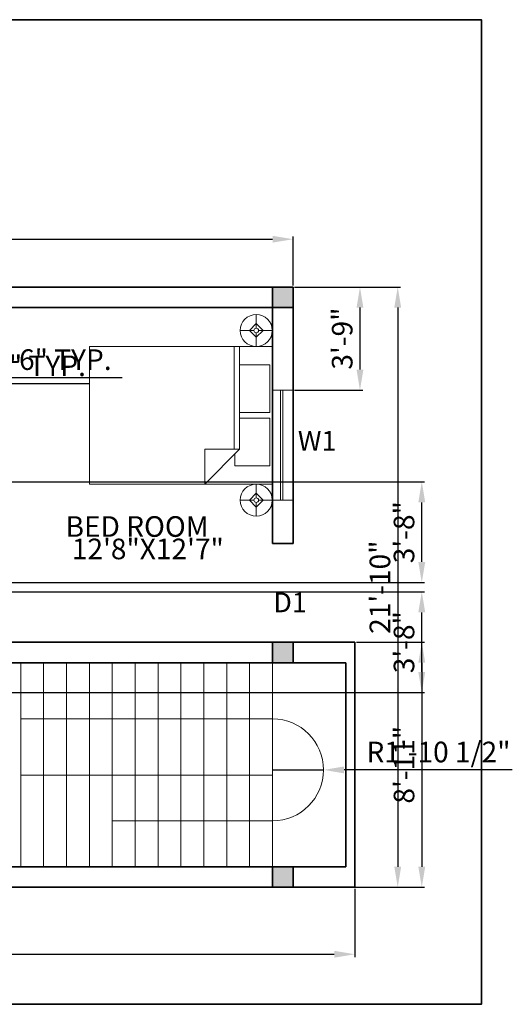
# Model space of a CAD drawing. Units: inches. Extents: x -281 to 2337, y 1647 to 2113.
# Tile 6 of 6: x 2121 to 2337, y 1674 to 2103. Entities that reach past the tile are written whole.
import ezdxf

# ---------------------------------------------------------------- set-up
doc = ezdxf.new("R2010")
doc.units = ezdxf.units.IN
for name, color, linetype, lineweight in [('A-ANNO-DIMS', 242, 'Continuous', 18), ('A-ANNO-IDEN', 11, 'Continuous', 18), ('A-ANNO-TTLB', 7, 'Continuous', 35), ('A-AREA-IDEN', 7, 'Continuous', 18), ('A-COLS', 1, 'Continuous', 35), ('A-FLOR-STRS', 7, 'Continuous', 18), ('A-FURN', 8, 'Continuous', 18), ('A-GLAZ', 3, 'Continuous', 18), ('A-WALL', 7, 'Continuous', 35)]:
    doc.layers.add(name, color=color, linetype=linetype, lineweight=lineweight)
doc.styles.get("Standard").update_dxf_attribs({"font": 'arial.ttf'})
doc.dimstyles.new('ISO-25', dxfattribs={"dimtxt": 9, "dimasz": 9, "dimexe": 1.25, "dimexo": 0.625, "dimgap": 2, "dimtad": 1, "dimdec": 1, "dimlunit": 4, "dimtxsty": 'Standard', "dimcen": 2.5, "dimadec": 0, "dimazin": 0, "dimtfac": 1, "dimtdec": 1, "dimtmove": 0, "dimatfit": 3, "dimfxl": 1, "dimarcsym": 0})

# ---------------------------------------------------------------- blocks, each defined once
blk = doc.blocks.new('Bed - Queen')
for p, q in [((0, -80.00003), (0, 0)), ((0, 0), (59.99999, 0)), ((59.99999, 0), (59.99999, -80.00003)), ((7.99999, -1.2), (28.79998, -1.2)), ((7.99999, -14.4), (7.99999, -1.2)), ((28.79998, -1.2), (28.79998, -14.4)), ((31.19999, -1.2), (51.99999, -1.2)), ((31.19999, -14.4), (31.19999, -1.2)), ((51.99999, -1.2), (51.99999, -16.4)), ((0, -14.4), (44.8, -14.4)), ((44.8, -16.8), (0, -16.8)), ((59.99999, -29.6), (44.8, -14.4)), ((44.8, -14.4), (44.8, -29.6)), ((51.99999, -16.4), (46.79936, -16.4)), ((44.8, -29.6), (59.99999, -29.6)), ((59.99999, -80.00003), (0, -80.00003))]:
    blk.add_line(p, q)
blk = doc.blocks.new('Lamp - Table')
for p, q in [((0, 7), (0, 1)), ((-1, 0), (-7, 0)), ((0, 3), (-3, 0)), ((-3, 0), (0, -3)), ((3, 0), (0, 3)), ((0, -3), (3, 0)), ((1, 0), (7, 0)), ((0, -1), (0, -7))]:
    blk.add_line(p, q)
for radius in [7, 1]:
    blk.add_circle((0, 0), radius)
blk = doc.blocks.new('*D10')
at = {"layer": 'A-ANNO-DIMS', "color": 0, "lineweight": -2, "transparency": 16777216}
for p, q in [((1746.88, 1987.41), (1746.88, 2008.91)), ((1755.88, 2007.66), (2231.88, 2007.66)), ((2240.88, 1987.41), (2240.88, 2008.91))]:
    blk.add_line(p, q, dxfattribs=at)
at = {"layer": 'A-ANNO-DIMS', "color": 0, "transparency": 16777216}
for points in [[(1755.88, 2009.16), (1755.88, 2006.16), (1746.88, 2007.66)], [(2231.88, 2009.16), (2231.88, 2006.16), (2240.88, 2007.66)]]:
    blk.add_solid(points, dxfattribs=at)
at = {"layer": 'Defpoints', "color": 0, "transparency": 16777216}
for p in [(2240.88, 2007.66), (1746.88, 1986.79), (2240.88, 1986.79)]:
    blk.add_point(p, dxfattribs=at)
at = {"layer": 'A-ANNO-DIMS', "color": 0, "transparency": 16777216, "insert": (1993.88, 2014.18), "char_height": 9, "attachment_point": 5}
blk.add_mtext('41\'-2"', dxfattribs=at)
blk = doc.blocks.new('*D11')
at = {"layer": 'A-ANNO-DIMS', "color": 0, "lineweight": -2, "transparency": 16777216}
for p, q in [((2241.51, 1986.79), (2287.82, 1986.79)), ((2286.57, 1977.79), (2286.57, 1733.79)), ((2241.51, 1724.79), (2287.82, 1724.79))]:
    blk.add_line(p, q, dxfattribs=at)
at = {"layer": 'A-ANNO-DIMS', "color": 0, "transparency": 16777216}
for points in [[(2285.07, 1977.79), (2288.07, 1977.79), (2286.57, 1986.79)], [(2285.07, 1733.79), (2288.07, 1733.79), (2286.57, 1724.79)]]:
    blk.add_solid(points, dxfattribs=at)
at = {"layer": 'Defpoints', "color": 0, "transparency": 16777216}
for p in [(2240.88, 1986.79), (2240.88, 1724.79), (2286.57, 1724.79)]:
    blk.add_point(p, dxfattribs=at)
at = {"layer": 'A-ANNO-DIMS', "color": 0, "transparency": 16777216, "insert": (2279.97, 1855.79), "char_height": 9, "attachment_point": 5, "rotation": 90}
blk.add_mtext('21\'-10"', dxfattribs=at)
blk = doc.blocks.new('COL-9x9')
h = blk.add_hatch(color=256)
h.dxf.hatch_style = 1
h.paths.add_polyline_path([(9, 9), (0, 9), (0, 0), (9, 0)])
for p, q in [((0, 9), (9, 9)), ((0, 0), (0, 9)), ((9, 9), (9, 0)), ((9, 0), (0, 0))]:
    blk.add_line(p, q)
blk = doc.blocks.new('WIN-W1-48')
for p, q in [((0, 48), (9, 48)), ((3.5, 0), (3.5, 48)), ((4.5, 0), (4.5, 48)), ((0, 0), (9, 0))]:
    blk.add_line(p, q)
blk = doc.blocks.new('*D31')
at = {"layer": 'A-ANNO-DIMS', "color": 0, "lineweight": -2, "transparency": 16777216}
for p, q in [((2020.54, 1951.16), (2020.54, 1946.04)), ((2050.54, 1951.16), (2050.54, 1946.04)), ((2029.54, 1947.29), (2041.54, 1947.29)), ((2050.54, 1947.29), (2166.14, 1947.29))]:
    blk.add_line(p, q, dxfattribs=at)
at = {"layer": 'A-ANNO-DIMS', "color": 0, "transparency": 16777216}
for points in [[(2029.54, 1948.79), (2029.54, 1945.79), (2020.54, 1947.29)], [(2041.54, 1948.79), (2041.54, 1945.79), (2050.54, 1947.29)]]:
    blk.add_solid(points, dxfattribs=at)
at = {"layer": 'Defpoints', "color": 0, "transparency": 16777216}
for p in [(2020.54, 1951.79), (2050.54, 1951.79), (2050.54, 1947.29)]:
    blk.add_point(p, dxfattribs=at)
at = {"layer": 'A-ANNO-DIMS', "color": 0, "transparency": 16777216, "insert": (2112.84, 1953.94), "char_height": 9, "attachment_point": 5}
blk.add_mtext('RANGE 2\'-6" TYP.', dxfattribs=at)
blk = doc.blocks.new('*D34')
at = {"layer": 'A-ANNO-DIMS', "color": 0, "lineweight": -2, "transparency": 16777216}
for p, q in [((2046.88, 1944.64), (2037.88, 1944.64)), ((2055.88, 1940.77), (2055.88, 1945.89)), ((2055.88, 1944.64), (2075.88, 1944.64)), ((2075.88, 1940.77), (2075.88, 1945.89)), ((2084.88, 1944.64), (2151.89, 1944.64))]:
    blk.add_line(p, q, dxfattribs=at)
at = {"layer": 'A-ANNO-DIMS', "color": 0, "transparency": 16777216}
for points in [[(2046.88, 1946.14), (2046.88, 1943.14), (2055.88, 1944.64)], [(2084.88, 1946.14), (2084.88, 1943.14), (2075.88, 1944.64)]]:
    blk.add_solid(points, dxfattribs=at)
at = {"layer": 'Defpoints', "color": 0, "transparency": 16777216}
for p in [(2075.88, 1944.64), (2055.88, 1940.14), (2075.88, 1940.14)]:
    blk.add_point(p, dxfattribs=at)
at = {"layer": 'A-ANNO-DIMS', "color": 0, "transparency": 16777216, "insert": (2122.89, 1951.24), "char_height": 9, "attachment_point": 5}
blk.add_mtext('1\'-8" TYP.', dxfattribs=at)
blk = doc.blocks.new('*D41')
at = {"layer": 'A-ANNO-DIMS', "color": 0, "lineweight": -2, "transparency": 16777216}
for p, q in [((1746.88, 1724.16), (1746.88, 1694.33)), ((2267.88, 1724.16), (2267.88, 1694.33)), ((1755.88, 1695.58), (2258.88, 1695.58))]:
    blk.add_line(p, q, dxfattribs=at)
at = {"layer": 'A-ANNO-DIMS', "color": 0, "transparency": 16777216}
for points in [[(1755.88, 1697.08), (1755.88, 1694.08), (1746.88, 1695.58)], [(2258.88, 1697.08), (2258.88, 1694.08), (2267.88, 1695.58)]]:
    blk.add_solid(points, dxfattribs=at)
at = {"layer": 'Defpoints', "color": 0, "transparency": 16777216}
for p in [(1746.88, 1724.79), (2267.88, 1724.79), (2267.88, 1695.58)]:
    blk.add_point(p, dxfattribs=at)
at = {"layer": 'A-ANNO-DIMS', "color": 0, "transparency": 16777216, "insert": (2007.38, 1702.18), "char_height": 9, "attachment_point": 5}
blk.add_mtext('43\'-5"', dxfattribs=at)
blk = doc.blocks.new('*D43')
at = {"layer": 'A-ANNO-DIMS', "color": 0, "lineweight": -2, "transparency": 16777216}
for p, q in [((2268.51, 1831.79), (2298.33, 1831.79)), ((2297.08, 1822.79), (2297.08, 1733.79)), ((2268.51, 1724.79), (2298.33, 1724.79))]:
    blk.add_line(p, q, dxfattribs=at)
at = {"layer": 'A-ANNO-DIMS', "color": 0, "transparency": 16777216}
for points in [[(2295.58, 1822.79), (2298.58, 1822.79), (2297.08, 1831.79)], [(2295.58, 1733.79), (2298.58, 1733.79), (2297.08, 1724.79)]]:
    blk.add_solid(points, dxfattribs=at)
at = {"layer": 'Defpoints', "color": 0, "transparency": 16777216}
for p in [(2267.88, 1831.79), (2267.88, 1724.79), (2297.08, 1724.79)]:
    blk.add_point(p, dxfattribs=at)
at = {"layer": 'A-ANNO-DIMS', "color": 0, "transparency": 16777216, "insert": (2290.49, 1778.29), "char_height": 9, "attachment_point": 5, "rotation": 90}
blk.add_mtext('8\'-11"', dxfattribs=at)
blk = doc.blocks.new('*D47')
at = {"layer": 'A-ANNO-DIMS', "color": 0, "lineweight": -2, "transparency": 16777216}
for p, q in [((2241.51, 1986.79), (2271.33, 1986.79)), ((2270.08, 1977.79), (2270.08, 1950.79)), ((2241.51, 1941.79), (2271.33, 1941.79))]:
    blk.add_line(p, q, dxfattribs=at)
at = {"layer": 'A-ANNO-DIMS', "color": 0, "transparency": 16777216}
for points in [[(2268.58, 1977.79), (2271.58, 1977.79), (2270.08, 1986.79)], [(2268.58, 1950.79), (2271.58, 1950.79), (2270.08, 1941.79)]]:
    blk.add_solid(points, dxfattribs=at)
at = {"layer": 'Defpoints', "color": 0, "transparency": 16777216}
for p in [(2240.88, 1986.79), (2240.88, 1941.79), (2270.08, 1941.79)]:
    blk.add_point(p, dxfattribs=at)
at = {"layer": 'A-ANNO-DIMS', "color": 0, "transparency": 16777216, "insert": (2263.48, 1964.29), "char_height": 9, "attachment_point": 5, "rotation": 90}
blk.add_mtext('3\'-9"', dxfattribs=at)
blk = doc.blocks.new('*D54')
at = {"layer": 'A-ANNO-DIMS', "color": 0, "lineweight": -2, "transparency": 16777216}
for p, q in [((1916.51, 1901.79), (2298.33, 1901.79)), ((2297.08, 1866.79), (2297.08, 1892.79)), ((1916.51, 1857.79), (2298.33, 1857.79))]:
    blk.add_line(p, q, dxfattribs=at)
at = {"layer": 'A-ANNO-DIMS', "color": 0, "transparency": 16777216}
for points in [[(2295.58, 1892.79), (2298.58, 1892.79), (2297.08, 1901.79)], [(2295.58, 1866.79), (2298.58, 1866.79), (2297.08, 1857.79)]]:
    blk.add_solid(points, dxfattribs=at)
at = {"layer": 'Defpoints', "color": 0, "transparency": 16777216}
for p in [(1915.88, 1901.79), (2297.08, 1901.79), (1915.88, 1857.79)]:
    blk.add_point(p, dxfattribs=at)
at = {"layer": 'A-ANNO-DIMS', "color": 0, "transparency": 16777216, "insert": (2290.48, 1879.79), "char_height": 9, "attachment_point": 5, "rotation": 90}
blk.add_mtext('3\'-8"', dxfattribs=at)
blk = doc.blocks.new('*D55')
at = {"layer": 'A-ANNO-DIMS', "color": 0, "lineweight": -2, "transparency": 16777216}
for p, q in [((1916.51, 1853.79), (2298.33, 1853.79)), ((2297.08, 1818.79), (2297.08, 1844.79)), ((1916.51, 1809.79), (2298.33, 1809.79))]:
    blk.add_line(p, q, dxfattribs=at)
at = {"layer": 'A-ANNO-DIMS', "color": 0, "transparency": 16777216}
for points in [[(2295.58, 1844.79), (2298.58, 1844.79), (2297.08, 1853.79)], [(2295.58, 1818.79), (2298.58, 1818.79), (2297.08, 1809.79)]]:
    blk.add_solid(points, dxfattribs=at)
at = {"layer": 'Defpoints', "color": 0, "transparency": 16777216}
for p in [(1915.88, 1853.79), (2297.08, 1853.79), (1915.88, 1809.79)]:
    blk.add_point(p, dxfattribs=at)
at = {"layer": 'A-ANNO-DIMS', "color": 0, "transparency": 16777216, "insert": (2290.48, 1831.79), "char_height": 9, "attachment_point": 5, "rotation": 90}
blk.add_mtext('3\'-8"', dxfattribs=at)
blk = doc.blocks.new('*D69')
at = {"layer": 'A-ANNO-DIMS', "color": 0, "lineweight": -2, "transparency": 16777216}
for p, q in [((2231.88, 1776.04), (2254.13, 1776.04)), ((2336.63, 1776.04), (2263.13, 1776.04))]:
    blk.add_line(p, q, dxfattribs=at)
at = {"layer": 'A-ANNO-DIMS', "color": 0, "transparency": 16777216}
blk.add_solid([(2263.13, 1777.54), (2263.13, 1774.54), (2254.13, 1776.04)], dxfattribs=at)
at = {"layer": 'Defpoints', "color": 0, "transparency": 16777216}
for p in [(2231.88, 1776.04), (2254.13, 1776.04)]:
    blk.add_point(p, dxfattribs=at)
at = {"layer": 'A-ANNO-DIMS', "color": 0, "transparency": 16777216, "insert": (2304.38, 1782.69), "char_height": 9, "attachment_point": 5, "rotation": 359.9992}
blk.add_mtext('R1\'-10 1/2"', dxfattribs=at)

msp = doc.modelspace()

# ---------------------------------------------------------------- linework, layer by layer
at = {"layer": 'A-ANNO-TTLB'}
msp.add_lwpolyline([(1037.79, 2103.48), (2323.1, 2103.48), (2323.1, 1673.73), (1037.79, 1673.73)], close=True, dxfattribs=at)
at = {"layer": 'A-FLOR-STRS'}
for p, q in [((2121.88, 1733.79), (2121.88, 1822.79)), ((2131.88, 1733.79), (2131.88, 1822.79)), ((2141.88, 1733.79), (2141.88, 1822.79)), ((2151.88, 1733.79), (2151.88, 1822.79)), ((2161.88, 1733.79), (2161.88, 1822.79)), ((2171.88, 1733.79), (2171.88, 1822.79)), ((2181.88, 1733.79), (2181.88, 1822.79)), ((2191.88, 1733.79), (2191.88, 1822.79)), ((2201.88, 1733.79), (2201.88, 1822.79)), ((2211.88, 1733.79), (2211.88, 1822.79)), ((2221.88, 1733.79), (2221.88, 1822.79)), ((2231.88, 1798.29), (2231.88, 1822.79)), ((2231.88, 1798.29), (2121.88, 1798.29)), ((2231.88, 1724.79), (2231.88, 1798.29)), ((2231.88, 1773.79), (2121.88, 1773.79)), ((2231.88, 1753.79), (2161.88, 1753.79))]:
    msp.add_line(p, q, dxfattribs=at)
msp.add_arc((2231.88, 1776.04), 22.25, 270, 90, dxfattribs=at)
at = {"layer": 'A-WALL'}
for p, q in [((1746.88, 1986.79), (2240.88, 1986.79)), ((2231.88, 1874.79), (2231.88, 1986.79)), ((2240.88, 1874.79), (2240.88, 1986.79)), ((1997.88, 1977.79), (2240.88, 1977.79)), ((2231.88, 1874.79), (2240.88, 1874.79)), ((2070.88, 1831.79), (2267.88, 1831.79)), ((2231.88, 1822.79), (2231.88, 1831.79)), ((2240.88, 1822.79), (2240.88, 1831.79)), ((2267.88, 1724.79), (2267.88, 1831.79)), ((2079.88, 1822.79), (2263.88, 1822.79)), ((2263.88, 1733.79), (2263.88, 1822.79)), ((2263.88, 1733.79), (1915.88, 1733.79)), ((2240.88, 1724.79), (2240.88, 1733.79)), ((2267.88, 1724.79), (1746.88, 1724.79))]:
    msp.add_line(p, q, dxfattribs=at)

# ---------------------------------------------------------------- block references
at = {"layer": 'A-COLS'}
for p in [(2231.88, 1977.79), (2231.88, 1822.79), (2231.88, 1724.79)]:
    msp.add_blockref('COL-9x9', p, dxfattribs=at)
at = {"layer": 'A-FURN'}
for p in [(2224.77, 1967.84), (2224.77, 1893.77)]:
    msp.add_blockref('Lamp - Table', p, dxfattribs=at)
at = {"layer": 'A-FURN', "rotation": 270}
msp.add_blockref('Bed - Queen', (2231.88, 1960.79), dxfattribs=at)
at = {"layer": 'A-GLAZ'}
msp.add_blockref('WIN-W1-48', (2231.88, 1893.79), dxfattribs=at)

# ---------------------------------------------------------------- texts
at = {"layer": 'A-ANNO-IDEN'}
for s, p in [('W1', (2242.94, 1915.39)), ('D1', (2232.24, 1844.84))]:
    msp.add_text(s, height=8.623, dxfattribs=at).set_placement(p)
at = {"layer": 'A-AREA-IDEN'}
for s, p in [('BED ROOM ', (2141.47, 1877.77)), (' 12\'8"X12\'7"', (2141.47, 1867.98))]:
    msp.add_text(s, height=9, dxfattribs=at).set_placement(p)

# ---------------------------------------------------------------- dimensions: what is measured, and where the dimension line sits
at = {"layer": 'A-ANNO-DIMS'}
for base, p1, p2, override, picture, middle in [((2240.88, 2007.66), (1746.88, 1986.79), (2240.88, 1986.79), {"dimclrd": 0, "dimclre": 0, "dimclrt": 0}, '*D10', (1993.88, 2014.18)), ((2267.88, 1695.58), (1746.88, 1724.79), (2267.88, 1724.79), {"dimdec": 1, "dimlfac": 1, "dimrnd": 0, "dimzin": 1, "dimdsep": 46, "dimlunit": 4, "dimfrac": 2}, '*D41', (2007.38, 1702.18))]:
    dim = msp.add_linear_dim(base=base, p1=p1, p2=p2, dimstyle='ISO-25', override=override, dxfattribs=at)
    dim.commit()
    dim.dimension.update_dxf_attribs({"geometry": picture, "text_midpoint": middle})
for base, p1, p2, angle, override, picture, middle in [((2286.57, 1724.79), (2240.88, 1986.79), (2240.88, 1724.79), 90, {"dimclrd": 0, "dimclre": 0, "dimclrt": 0}, '*D11', (2279.97, 1855.79)), ((2270.08, 1941.79), (2240.88, 1986.79), (2240.88, 1941.79), 270, {"dimdec": 1, "dimlfac": 1, "dimrnd": 0, "dimzin": 1, "dimdsep": 46, "dimlunit": 4, "dimfrac": 2}, '*D47', (2263.48, 1964.29)), ((2297.08, 1901.79), (1915.88, 1857.79), (1915.88, 1901.79), 90, {"dimdec": 1, "dimlfac": 1, "dimrnd": 0, "dimzin": 1, "dimdsep": 46, "dimlunit": 4, "dimfrac": 2}, '*D54', (2290.48, 1879.79)), ((2297.08, 1853.79), (1915.88, 1809.79), (1915.88, 1853.79), 90, {"dimdec": 1, "dimlfac": 1, "dimrnd": 0, "dimzin": 1, "dimdsep": 46, "dimlunit": 4, "dimfrac": 2}, '*D55', (2290.48, 1831.79)), ((2297.08, 1724.79), (2267.88, 1831.79), (2267.88, 1724.79), 270, {"dimdec": 1, "dimlfac": 1, "dimrnd": 0, "dimzin": 1, "dimdsep": 46, "dimlunit": 4, "dimfrac": 2}, '*D43', (2290.49, 1778.29))]:
    dim = msp.add_linear_dim(base=base, p1=p1, p2=p2, angle=angle, dimstyle='ISO-25', override=override, dxfattribs=at)
    dim.commit()
    dim.dimension.update_dxf_attribs({"geometry": picture, "text_midpoint": middle})
for base, p1, p2, text, picture, middle in [((2050.54, 1947.29), (2020.54, 1951.79), (2050.54, 1951.79), 'RANGE <> TYP.', '*D31', (2112.84, 1953.94)), ((2075.88, 1944.64), (2055.88, 1940.14), (2075.88, 1940.14), '<> TYP.', '*D34', (2122.89, 1951.24))]:
    dim = msp.add_linear_dim(base=base, p1=p1, p2=p2, text=text, dimstyle='ISO-25', override={"dimdec": 1, "dimlfac": 1, "dimrnd": 0, "dimzin": 1, "dimdsep": 46, "dimlunit": 4, "dimfrac": 2}, dxfattribs=at)
    dim.commit()
    dim.dimension.update_dxf_attribs({"geometry": picture, "text_midpoint": middle})
dim = msp.add_radius_dim(center=(2231.880179, 1776.038328), mpoint=(2254.130179, 1776.038), dimstyle='ISO-25', override={"dimdec": 1, "dimlfac": 1, "dimrnd": 0, "dimzin": 1, "dimdsep": 46, "dimlunit": 4, "dimfrac": 2}, dxfattribs=at)
dim.commit()
dim.dimension.update_dxf_attribs({"geometry": '*D69', "text_midpoint": (2304.38095921, 1782.69073808)})

doc.saveas('drawing.dxf')
